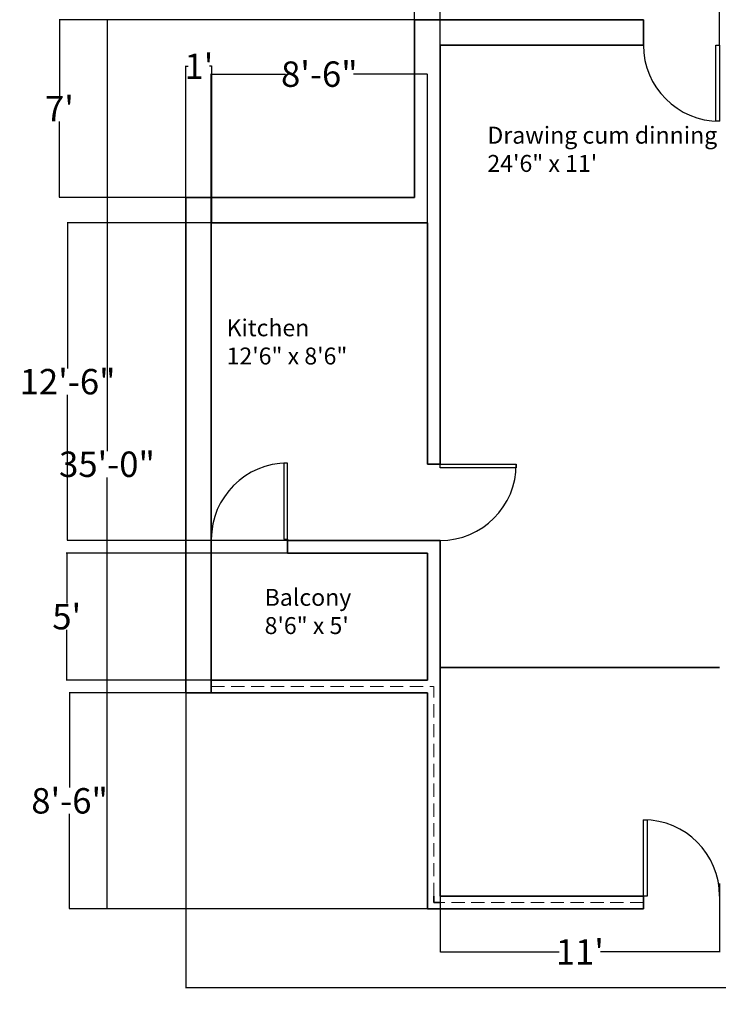
# Model space of a CAD drawing. Units: inches. Extents: x 2450 to 4494, y 1482 to 2597.
# Tile 1 of 7: x 2450 to 2780, y 1722 to 2188. Entities that reach past the tile are written whole.
import ezdxf

# ---------------------------------------------------------------- set-up
doc = ezdxf.new("R2010")
doc.units = ezdxf.units.IN
doc.header["$LTSCALE"] = 5
doc.header["$MEASUREMENT"] = 0
doc.linetypes.add('HIDDEN', pattern=[0.375, 0.25, -0.125])
for name, color, linetype, lineweight in [('A-ANNO-DIMS', 2, 'Continuous', 18), ('A-AREA-IDEN', 7, 'Continuous', 18), ('A-DOOR', 4, 'Continuous', 25), ('A-WALL', 7, 'Continuous', 35), ('A-WALL-HIDN', 7, 'HIDDEN', 18)]:
    doc.layers.add(name, color=color, linetype=linetype, lineweight=lineweight)
doc.styles.get("Standard").update_dxf_attribs({"font": 'arial.ttf'})
doc.dimstyles.get("Standard").update_dxf_attribs({"dimtxt": 12, "dimasz": 0.18, "dimexe": 0.18, "dimexo": 0.0625, "dimgap": 0.09, "dimtad": 0, "dimtih": 1, "dimtoh": 1, "dimdec": 0, "dimzin": 0, "dimdsep": 46, "dimlunit": 3, "dimtxsty": 'Standard', "dimcen": 0.09, "dimadec": 0, "dimazin": 0, "dimtfac": 1, "dimtdec": 0, "dimtofl": 0, "dimtmove": 0, "dimatfit": 3, "dimfxl": 1, "dimtolj": 1, "dimtzin": 0, "dimarcsym": 0})

# ---------------------------------------------------------------- blocks, each defined once
blk = doc.blocks.new('*U4')
for p, q in [((-36, 0), (-36, -6)), ((0, 0), (0, -6))]:
    blk.add_line(p, q)
blk.add_lwpolyline([(0, 0), (0, 36), (-1.75, 36), (-1.75, 0)], close=True)
blk.add_arc((0, 0), 36, 90, 180)
blk = doc.blocks.new('*U2')
for p, q in [((0, 0), (0, -6)), ((36, 0), (36, -6))]:
    blk.add_line(p, q)
blk.add_lwpolyline([(0, 0), (0, 36), (1.75, 36), (1.75, 0)], close=True)
blk.add_arc((0, 0), 36, 0, 90)
blk = doc.blocks.new('*U5')
for p, q in [((-36, 0), (-36, 6)), ((0, 0), (0, 6))]:
    blk.add_line(p, q)
blk.add_lwpolyline([(0, 0), (0, -36), (-1.75, -36), (-1.75, 0)], close=True)
blk.add_arc((0, 0), 36, 180, 270)
blk = doc.blocks.new('*D10')
at = {"layer": 'A-ANNO-DIMS', "color": 0, "lineweight": -2, "ltscale": 5, "transparency": 16777216}
for p, q in [((2648.93, 2175.63), (2648.93, 2236.37)), ((2649.11, 2236.19), (2705.22, 2236.19)), ((2780.75, 2236.19), (2724.64, 2236.19)), ((2780.93, 2175.63), (2780.93, 2236.37))]:
    blk.add_line(p, q, dxfattribs=at)
at = {"layer": 'A-ANNO-DIMS', "color": 0, "ltscale": 5, "transparency": 16777216}
for points in [[(2649.11, 2236.22), (2649.11, 2236.16), (2648.93, 2236.19)], [(2780.75, 2236.22), (2780.75, 2236.16), (2780.93, 2236.19)]]:
    blk.add_solid(points, dxfattribs=at)
at = {"layer": 'Defpoints', "color": 0, "ltscale": 5, "transparency": 16777216}
for p in [(2780.93, 2236.19), (2648.93, 2175.57), (2780.93, 2175.57)]:
    blk.add_point(p, dxfattribs=at)
at = {"layer": 'A-ANNO-DIMS', "color": 0, "ltscale": 5, "transparency": 16777216, "insert": (2714.93, 2236.19), "char_height": 12, "attachment_point": 5}
blk.add_mtext("\\A1;11'", dxfattribs=at)
blk = doc.blocks.new('*D11')
at = {"layer": 'A-ANNO-DIMS', "color": 0, "lineweight": -2, "ltscale": 5, "transparency": 16777216}
for p, q in [((2636.93, 2175.63), (2636.93, 2235.95)), ((2637.11, 2235.77), (2637.88, 2235.77)), ((2648.75, 2235.77), (2647.98, 2235.77)), ((2648.93, 2175.63), (2648.93, 2235.95))]:
    blk.add_line(p, q, dxfattribs=at)
at = {"layer": 'A-ANNO-DIMS', "color": 0, "ltscale": 5, "transparency": 16777216}
for points in [[(2637.11, 2235.8), (2637.11, 2235.74), (2636.93, 2235.77)], [(2648.75, 2235.8), (2648.75, 2235.74), (2648.93, 2235.77)]]:
    blk.add_solid(points, dxfattribs=at)
at = {"layer": 'Defpoints', "color": 0, "ltscale": 5, "transparency": 16777216}
for p in [(2636.93, 2235.77), (2636.93, 2175.57), (2648.93, 2175.57)]:
    blk.add_point(p, dxfattribs=at)
at = {"layer": 'A-ANNO-DIMS', "color": 0, "ltscale": 5, "transparency": 16777216, "insert": (2642.93, 2235.77), "char_height": 12, "attachment_point": 5}
blk.add_mtext("\\A1;1'", dxfattribs=at)
blk = doc.blocks.new('*D12')
at = {"layer": 'A-ANNO-DIMS', "color": 0, "lineweight": -2, "ltscale": 5, "transparency": 16777216}
for p, q in [((2540.93, 2091.63), (2540.93, 2162.03)), ((2541.11, 2161.85), (2575.88, 2161.85)), ((2642.75, 2161.85), (2607.98, 2161.85)), ((2642.93, 2091.63), (2642.93, 2162.03))]:
    blk.add_line(p, q, dxfattribs=at)
at = {"layer": 'A-ANNO-DIMS', "color": 0, "ltscale": 5, "transparency": 16777216}
for points in [[(2541.11, 2161.88), (2541.11, 2161.82), (2540.93, 2161.85)], [(2642.75, 2161.88), (2642.75, 2161.82), (2642.93, 2161.85)]]:
    blk.add_solid(points, dxfattribs=at)
at = {"layer": 'Defpoints', "color": 0, "ltscale": 5, "transparency": 16777216}
for p in [(2540.93, 2161.85), (2540.93, 2091.57), (2642.93, 2091.57)]:
    blk.add_point(p, dxfattribs=at)
at = {"layer": 'A-ANNO-DIMS', "color": 0, "ltscale": 5, "transparency": 16777216, "insert": (2591.93, 2161.85), "char_height": 12, "attachment_point": 5}
blk.add_mtext('\\A1;8\'-6"', dxfattribs=at)
blk = doc.blocks.new('*D13')
at = {"layer": 'A-ANNO-DIMS', "color": 0, "lineweight": -2, "ltscale": 5, "transparency": 16777216}
for p, q in [((2528.93, 2091.63), (2528.93, 2165.72)), ((2529.11, 2165.54), (2530.02, 2165.54)), ((2541.02, 2165.54), (2540.11, 2165.54)), ((2541.2, 2091.63), (2541.2, 2165.72))]:
    blk.add_line(p, q, dxfattribs=at)
at = {"layer": 'A-ANNO-DIMS', "color": 0, "ltscale": 5, "transparency": 16777216}
for points in [[(2529.11, 2165.57), (2529.11, 2165.51), (2528.93, 2165.54)], [(2541.02, 2165.57), (2541.02, 2165.51), (2541.2, 2165.54)]]:
    blk.add_solid(points, dxfattribs=at)
at = {"layer": 'Defpoints', "color": 0, "ltscale": 5, "transparency": 16777216}
for p in [(2528.93, 2165.54), (2528.93, 2091.57), (2541.2, 2091.57)]:
    blk.add_point(p, dxfattribs=at)
at = {"layer": 'A-ANNO-DIMS', "color": 0, "ltscale": 5, "transparency": 16777216, "insert": (2535.07, 2165.54), "char_height": 12, "attachment_point": 5}
blk.add_mtext("\\A1;1'", dxfattribs=at)
blk = doc.blocks.new('*D14')
at = {"layer": 'A-ANNO-DIMS', "color": 0, "lineweight": -2, "ltscale": 5, "transparency": 16777216}
for p, q in [((2576.87, 2091.57), (2472.9, 2091.57)), ((2473.08, 2091.39), (2473.08, 2022.79)), ((2473.08, 1941.75), (2473.08, 2010.35)), ((2576.87, 1941.57), (2472.9, 1941.57))]:
    blk.add_line(p, q, dxfattribs=at)
at = {"layer": 'A-ANNO-DIMS', "color": 0, "ltscale": 5, "transparency": 16777216}
for points in [[(2473.05, 2091.39), (2473.11, 2091.39), (2473.08, 2091.57)], [(2473.05, 1941.75), (2473.11, 1941.75), (2473.08, 1941.57)]]:
    blk.add_solid(points, dxfattribs=at)
at = {"layer": 'Defpoints', "color": 0, "ltscale": 5, "transparency": 16777216}
for p in [(2473.08, 2091.57), (2576.93, 2091.57), (2576.93, 1941.57)]:
    blk.add_point(p, dxfattribs=at)
at = {"layer": 'A-ANNO-DIMS', "color": 0, "ltscale": 5, "transparency": 16777216, "insert": (2473.08, 2016.57), "char_height": 12, "attachment_point": 5}
blk.add_mtext('\\A1;12\'-6"', dxfattribs=at)
blk = doc.blocks.new('*D15')
at = {"layer": 'A-ANNO-DIMS', "color": 0, "lineweight": -2, "ltscale": 5, "transparency": 16777216}
for p, q in [((2636.87, 2187.57), (2469.05, 2187.57)), ((2469.23, 2187.39), (2469.23, 2151.66)), ((2469.23, 2103.75), (2469.23, 2139.48)), ((2636.87, 2103.57), (2469.05, 2103.57))]:
    blk.add_line(p, q, dxfattribs=at)
at = {"layer": 'A-ANNO-DIMS', "color": 0, "ltscale": 5, "transparency": 16777216}
for points in [[(2469.2, 2187.39), (2469.26, 2187.39), (2469.23, 2187.57)], [(2469.2, 2103.75), (2469.26, 2103.75), (2469.23, 2103.57)]]:
    blk.add_solid(points, dxfattribs=at)
at = {"layer": 'Defpoints', "color": 0, "ltscale": 5, "transparency": 16777216}
for p in [(2636.93, 2187.57), (2469.23, 2103.57), (2636.93, 2103.57)]:
    blk.add_point(p, dxfattribs=at)
at = {"layer": 'A-ANNO-DIMS', "color": 0, "ltscale": 5, "transparency": 16777216, "insert": (2469.23, 2145.57), "char_height": 12, "attachment_point": 5}
blk.add_mtext("\\A1;7'", dxfattribs=at)
blk = doc.blocks.new('*D16')
at = {"layer": 'A-ANNO-DIMS', "color": 0, "lineweight": -2, "ltscale": 5, "transparency": 16777216}
for p, q in [((2576.87, 1935.57), (2472.47, 1935.57)), ((2472.65, 1935.39), (2472.65, 1911.76)), ((2472.65, 1875.75), (2472.65, 1899.38)), ((2576.87, 1875.57), (2472.47, 1875.57))]:
    blk.add_line(p, q, dxfattribs=at)
at = {"layer": 'A-ANNO-DIMS', "color": 0, "ltscale": 5, "transparency": 16777216}
for points in [[(2472.62, 1935.39), (2472.68, 1935.39), (2472.65, 1935.57)], [(2472.62, 1875.75), (2472.68, 1875.75), (2472.65, 1875.57)]]:
    blk.add_solid(points, dxfattribs=at)
at = {"layer": 'Defpoints', "color": 0, "ltscale": 5, "transparency": 16777216}
for p in [(2576.93, 1935.57), (2472.65, 1875.57), (2576.93, 1875.57)]:
    blk.add_point(p, dxfattribs=at)
at = {"layer": 'A-ANNO-DIMS', "color": 0, "ltscale": 5, "transparency": 16777216, "insert": (2472.65, 1905.57), "char_height": 12, "attachment_point": 5}
blk.add_mtext("\\A1;5'", dxfattribs=at)
blk = doc.blocks.new('*D17')
at = {"layer": 'A-ANNO-DIMS', "color": 0, "lineweight": -2, "ltscale": 5, "transparency": 16777216}
for p, q in [((2642.87, 1869.57), (2473.83, 1869.57)), ((2474.01, 1869.39), (2474.01, 1824.79)), ((2474.01, 1767.75), (2474.01, 1812.35)), ((2642.87, 1767.57), (2473.83, 1767.57))]:
    blk.add_line(p, q, dxfattribs=at)
at = {"layer": 'A-ANNO-DIMS', "color": 0, "ltscale": 5, "transparency": 16777216}
for points in [[(2473.98, 1869.39), (2474.04, 1869.39), (2474.01, 1869.57)], [(2473.98, 1767.75), (2474.04, 1767.75), (2474.01, 1767.57)]]:
    blk.add_solid(points, dxfattribs=at)
at = {"layer": 'Defpoints', "color": 0, "ltscale": 5, "transparency": 16777216}
for p in [(2642.93, 1869.57), (2474.01, 1767.57), (2642.93, 1767.57)]:
    blk.add_point(p, dxfattribs=at)
at = {"layer": 'A-ANNO-DIMS', "color": 0, "ltscale": 5, "transparency": 16777216, "insert": (2474.01, 1818.57), "char_height": 12, "attachment_point": 5}
blk.add_mtext('\\A1;8\'-6"', dxfattribs=at)
blk = doc.blocks.new('*D18')
at = {"layer": 'A-ANNO-DIMS', "color": 0, "lineweight": -2, "ltscale": 5, "transparency": 16777216}
for p, q in [((2648.93, 1779.51), (2648.93, 1747)), ((2780.93, 1779.51), (2780.93, 1747)), ((2649.11, 1747.18), (2705.22, 1747.18)), ((2780.75, 1747.18), (2724.64, 1747.18))]:
    blk.add_line(p, q, dxfattribs=at)
at = {"layer": 'A-ANNO-DIMS', "color": 0, "ltscale": 5, "transparency": 16777216}
for points in [[(2649.11, 1747.21), (2649.11, 1747.15), (2648.93, 1747.18)], [(2780.75, 1747.21), (2780.75, 1747.15), (2780.93, 1747.18)]]:
    blk.add_solid(points, dxfattribs=at)
at = {"layer": 'Defpoints', "color": 0, "ltscale": 5, "transparency": 16777216}
for p in [(2648.93, 1779.57), (2780.93, 1779.57), (2648.93, 1747.18)]:
    blk.add_point(p, dxfattribs=at)
at = {"layer": 'A-ANNO-DIMS', "color": 0, "ltscale": 5, "transparency": 16777216, "insert": (2714.93, 1747.18), "char_height": 12, "attachment_point": 5}
blk.add_mtext("\\A1;11'", dxfattribs=at)
blk = doc.blocks.new('*D69')
at = {"layer": 'A-ANNO-DIMS', "color": 0, "lineweight": -2, "ltscale": 5, "transparency": 16777216}
for p, q in [((2528.93, 1869.51), (2528.93, 1730.14)), ((3092.93, 1863.51), (3092.93, 1730.14)), ((2529.11, 1730.32), (2789.99, 1730.32)), ((3092.75, 1730.32), (2831.87, 1730.32))]:
    blk.add_line(p, q, dxfattribs=at)
at = {"layer": 'A-ANNO-DIMS', "color": 0, "ltscale": 5, "transparency": 16777216}
for points in [[(2529.11, 1730.35), (2529.11, 1730.29), (2528.93, 1730.32)], [(3092.75, 1730.35), (3092.75, 1730.29), (3092.93, 1730.32)]]:
    blk.add_solid(points, dxfattribs=at)
at = {"layer": 'Defpoints', "color": 0, "ltscale": 5, "transparency": 16777216}
for p in [(2528.93, 1869.57), (3092.93, 1863.57), (3092.93, 1730.32)]:
    blk.add_point(p, dxfattribs=at)
at = {"layer": 'A-ANNO-DIMS', "color": 0, "ltscale": 5, "transparency": 16777216, "insert": (2810.93, 1730.32), "char_height": 12, "attachment_point": 5}
blk.add_mtext('\\A1;47\'-0"', dxfattribs=at)
blk = doc.blocks.new('*D70')
at = {"layer": 'A-ANNO-DIMS', "color": 0, "lineweight": -2, "ltscale": 5, "transparency": 16777216}
for p, q in [((2636.87, 2187.57), (2491.5, 2187.57)), ((2491.68, 2187.39), (2491.68, 1983.79)), ((2491.68, 1767.75), (2491.68, 1971.35)), ((2642.87, 1767.57), (2491.5, 1767.57))]:
    blk.add_line(p, q, dxfattribs=at)
at = {"layer": 'A-ANNO-DIMS', "color": 0, "ltscale": 5, "transparency": 16777216}
for points in [[(2491.65, 2187.39), (2491.71, 2187.39), (2491.68, 2187.57)], [(2491.65, 1767.75), (2491.71, 1767.75), (2491.68, 1767.57)]]:
    blk.add_solid(points, dxfattribs=at)
at = {"layer": 'Defpoints', "color": 0, "ltscale": 5, "transparency": 16777216}
for p in [(2636.93, 2187.57), (2491.68, 1767.57), (2642.93, 1767.57)]:
    blk.add_point(p, dxfattribs=at)
at = {"layer": 'A-ANNO-DIMS', "color": 0, "ltscale": 5, "transparency": 16777216, "insert": (2491.68, 1977.57), "char_height": 12, "attachment_point": 5}
blk.add_mtext('\\A1;35\'-0"', dxfattribs=at)

msp = doc.modelspace()

# ---------------------------------------------------------------- linework, layer by layer
at = {"layer": 'A-WALL'}
for p, q in [((2636.93, 2175.57), (2636.93, 2187.57)), ((2744.93, 2187.57), (2636.93, 2187.57)), ((2744.93, 2175.57), (2744.93, 2187.57)), ((2636.93, 2175.57), (2636.93, 2103.57)), ((2648.93, 2175.57), (2648.93, 1977.57)), ((2744.93, 2175.57), (2648.93, 2175.57)), ((2528.93, 2103.57), (2528.93, 1869.57)), ((2540.93, 2103.57), (2528.93, 2103.57)), ((2636.93, 2103.57), (2540.93, 2103.57)), ((2540.93, 2091.57), (2540.93, 1941.57)), ((2642.93, 2091.57), (2540.93, 2091.57)), ((2642.93, 2091.57), (2642.93, 1977.57)), ((2642.93, 1977.57), (2648.93, 1977.57)), ((2540.93, 1941.57), (2540.93, 1935.57)), ((2642.93, 1941.57), (2576.93, 1941.57)), ((2576.93, 1941.57), (2576.93, 1935.57)), ((2642.93, 1941.57), (2648.93, 1941.57)), ((2648.93, 1941.57), (2648.93, 1773.57)), ((2540.93, 1935.57), (2540.93, 1875.57)), ((2642.93, 1935.57), (2576.93, 1935.57)), ((2642.93, 1935.57), (2642.93, 1875.57)), ((2780.93, 1881.57), (2648.93, 1881.57)), ((2642.93, 1875.57), (2540.93, 1875.57)), ((2540.93, 1875.57), (2540.93, 1869.57)), ((2540.93, 1869.57), (2528.93, 1869.57)), ((2642.93, 1869.57), (2540.93, 1869.57)), ((2642.93, 1869.57), (2642.93, 1779.57)), ((2642.93, 1779.57), (2642.93, 1767.57)), ((2645.93, 1773.57), (2645.93, 1770.57)), ((2648.93, 1773.57), (2744.93, 1773.57)), ((2744.93, 1773.57), (2744.93, 1767.57)), ((2642.93, 1767.57), (2744.93, 1767.57)), ((2648.93, 1770.57), (2645.93, 1770.57))]:
    msp.add_line(p, q, dxfattribs=at)
at = {"layer": 'A-WALL-HIDN', "ltscale": 5}
for p, q in [((2540.93, 1872.57), (2645.88, 1872.57)), ((2645.93, 1773.57), (2645.93, 1872.57)), ((2744.93, 1770.57), (2648.93, 1770.57))]:
    msp.add_line(p, q, dxfattribs=at)

# ---------------------------------------------------------------- block references
at = {"layer": 'A-DOOR'}
for name, p in [('*U5', (2780.93, 2175.57)), ('*U4', (2576.93, 1942.1)), ('*U2', (2744.93, 1773.57))]:
    msp.add_blockref(name, p, dxfattribs=at)
at = {"layer": 'A-DOOR', "rotation": 270}
msp.add_blockref('*U2', (2648.93, 1977.57), dxfattribs=at)

# ---------------------------------------------------------------- texts
at = {"layer": 'A-AREA-IDEN', "char_height": 8, "attachment_point": 1}
for s, insert in [('Drawing cum dinning\\P24\'6" x 11\'', (2671.26, 2137.01)), ('Kitchen\\P12\'6" x 8\'6"', (2548.13, 2046.03)), ('Balcony\\P8\'6" x 5\'', (2566.08, 1918.69))]:
    msp.add_mtext_dynamic_manual_height_columns(s, width=155.5618, gutter_width=1, heights=[0], dxfattribs=dict(at, insert=insert))

# ---------------------------------------------------------------- dimensions: what is measured, and where the dimension line sits
at = {"layer": 'A-ANNO-DIMS', "ltscale": 5}
for base, p1, p2, override, picture, middle in [((2636.93, 2235.77), (2648.93, 2175.57), (2636.93, 2175.57), {"dimclrd": 0, "dimclre": 0, "dimclrt": 0}, '*D11', (2642.93, 2235.77)), ((2780.93, 2236.19), (2648.93, 2175.57), (2780.93, 2175.57), {"dimclrd": 0, "dimclre": 0, "dimclrt": 0}, '*D10', (2714.93, 2236.19)), ((2528.93, 2165.54), (2541.2, 2091.57), (2528.93, 2091.57), {"dimclrd": 0, "dimclre": 0, "dimclrt": 0}, '*D13', (2535.07, 2165.54)), ((2540.93, 2161.85), (2642.93, 2091.57), (2540.93, 2091.57), {"dimclrd": 0, "dimclre": 0, "dimclrt": 0}, '*D12', (2591.93, 2161.85)), ((3092.93, 1730.32), (2528.93, 1869.57), (3092.93, 1863.57), {"dimdec": 1, "dimlfac": 1, "dimrnd": 0, "dimzin": 1, "dimdsep": 46, "dimlunit": 4, "dimfrac": 2}, '*D69', (2810.93, 1730.32)), ((2648.93, 1747.18), (2780.93, 1779.57), (2648.93, 1779.57), {"dimclrd": 0, "dimclre": 0, "dimclrt": 0}, '*D18', (2714.93, 1747.18))]:
    dim = msp.add_linear_dim(base=base, p1=p1, p2=p2, dimstyle='Standard', override=override, dxfattribs=at)
    dim.commit()
    dim.dimension.update_dxf_attribs({"geometry": picture, "text_midpoint": middle})
for base, p1, p2, override, picture, middle in [((2469.23, 2103.57), (2636.93, 2187.57), (2636.93, 2103.57), {"dimclrd": 0, "dimclre": 0, "dimclrt": 0}, '*D15', (2469.23, 2145.57)), ((2491.68, 1767.57), (2636.93, 2187.57), (2642.93, 1767.57), {"dimdec": 1, "dimlfac": 1, "dimrnd": 0, "dimzin": 1, "dimdsep": 46, "dimlunit": 4, "dimfrac": 2}, '*D70', (2491.68, 1977.57)), ((2473.08, 2091.57), (2576.93, 1941.57), (2576.93, 2091.57), {"dimclrd": 0, "dimclre": 0, "dimclrt": 0}, '*D14', (2473.08, 2016.57)), ((2472.65, 1875.57), (2576.93, 1935.57), (2576.93, 1875.57), {"dimclrd": 0, "dimclre": 0, "dimclrt": 0}, '*D16', (2472.65, 1905.57)), ((2474.01, 1767.57), (2642.93, 1869.57), (2642.93, 1767.57), {"dimclrd": 0, "dimclre": 0, "dimclrt": 0}, '*D17', (2474.01, 1818.57))]:
    dim = msp.add_linear_dim(base=base, p1=p1, p2=p2, angle=90, dimstyle='Standard', override=override, dxfattribs=at)
    dim.commit()
    dim.dimension.update_dxf_attribs({"geometry": picture, "text_midpoint": middle})

doc.saveas('drawing.dxf')
